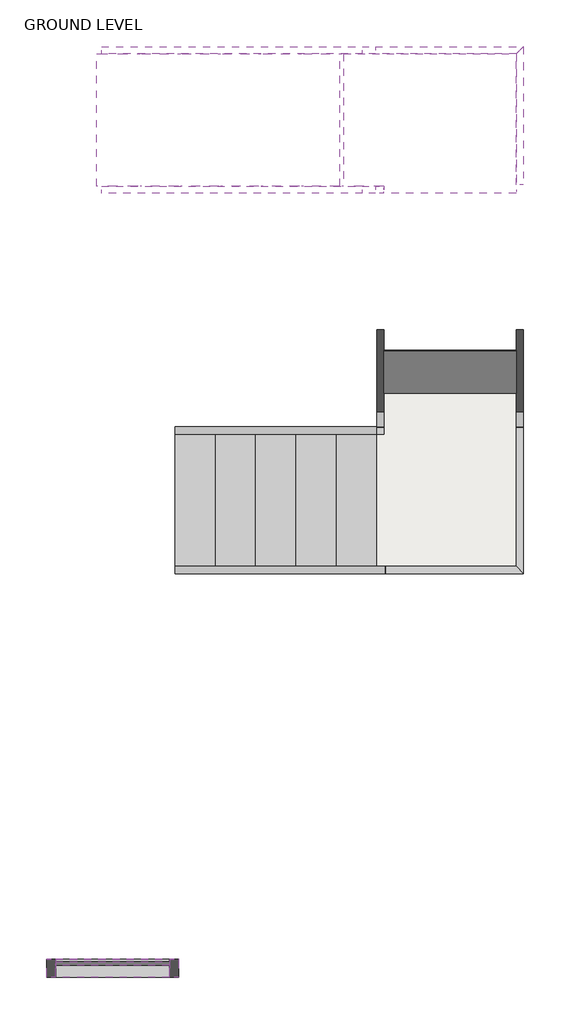
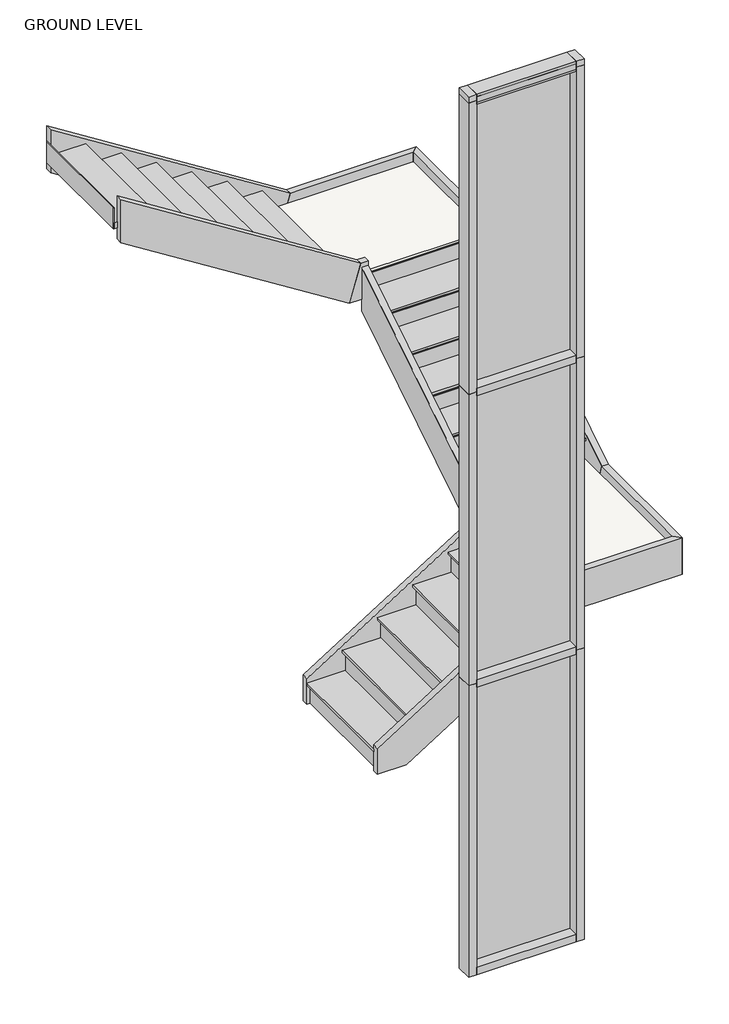
# One storey, incomplete: 25 members, 3 plates, 3 stair flights, 2 slabs.
"""IFC4 building model written with IfcOpenShell, lengths in millimetres."""

from ifc_helpers import new_model, si_unit, frame, origin, place, context, project, spatial, polyline, outline, extrude, faceted_brep, transform, mapped, element, save
from components import member_429f6687, member_18a184ad, member_ee409385, member_e0baf447, system_panel_glazed_7e875482, system_panel_glazed_4ec892b8, non_monolithic_landing_614a383d, non_monolithic_landing_589093d1, stair_flight_883e4480, stair_flight_150202ba, stair_flight_54ffcc7a

model = new_model("IFC4")

# Units and contexts
model_context = context("Model", 3, world=origin())
ifc_project = project(units=[si_unit("LENGTHUNIT", "METRE", prefix="MILLI")], contexts=[model_context])

# Site, building, storey
site = spatial("IfcSite", under=ifc_project)
building = spatial("IfcBuilding", under=site)
storey = spatial("IfcBuildingStorey", under=building, Name="GROUND LEVEL", Elevation=0.0)

# Members
placement = place(None, origin())
member_shape = member_429f6687(model_context)
element("IfcMember", 1, ObjectType="Rectangular Mullion : 2.5\" x 5\" rectangular", at=placement, inside=storey, context=model_context, shape_type="MappedRepresentation", body=[
    mapped(member_shape, transform((7470.37371, -13500.720363, 7669.779075), x_axis=(0.0, 0.0, 1.0), y_axis=(0.0, -1.0, 0.0), z_axis=(1.0, 0.0, 0.0))),
])
element("IfcMember", 2, ObjectType="Rectangular Mullion : 2.5\" x 5\" rectangular", at=placement, inside=storey, context=model_context, shape_type="MappedRepresentation", body=[
    mapped(member_shape, transform((6682.97371, -13500.720363, 304.8), x_axis=(0.0, 0.0, -1.0), y_axis=(0.0, -1.0, 0.0), z_axis=(-1.0, 0.0, 0.0))),
])
member_2_shape = member_18a184ad(model_context)
element("IfcMember", 3, ObjectType="Rectangular Mullion : 2.5\" x 5\" rectangular", at=placement, inside=storey, context=model_context, shape_type="MappedRepresentation", body=[
    mapped(member_2_shape, transform((7470.37371, -13500.720363, 2743.2), x_axis=(0.0, 0.0, 1.0), y_axis=(0.0, -1.0, 0.0), z_axis=(1.0, 0.0, 0.0))),
])
element("IfcMember", 4, ObjectType="Rectangular Mullion : 2.5\" x 5\" rectangular", at=placement, inside=storey, context=model_context, shape_type="MappedRepresentation", body=[
    mapped(member_2_shape, transform((7470.37371, -13500.720363, 5181.6), x_axis=(0.0, 0.0, 1.0), y_axis=(0.0, -1.0, 0.0), z_axis=(1.0, 0.0, 0.0))),
])
element("IfcMember", 5, ObjectType="Rectangular Mullion : 2.5\" x 5\" rectangular", at=placement, inside=storey, context=model_context, shape_type="MappedRepresentation", body=[
    mapped(member_2_shape, transform((7470.37371, -13500.720363, 7620.0), x_axis=(0.0, 0.0, 1.0), y_axis=(0.0, -1.0, 0.0), z_axis=(1.0, 0.0, 0.0))),
])
member_3_shape = member_ee409385(model_context)
element("IfcMember", 6, ObjectType="Rectangular Mullion : 2.5\" x 5\" rectangular", at=placement, inside=storey, context=model_context, shape_type="MappedRepresentation", body=[
    mapped(member_3_shape, transform((7533.87371, -13500.720363, 304.8), x_axis=(1.0, 0.0, 0.0), y_axis=(0.0, -1.0, 0.0), z_axis=(0.0, 0.0, -1.0))),
])
element("IfcMember", 7, ObjectType="Rectangular Mullion : 2.5\" x 5\" rectangular", at=placement, inside=storey, context=model_context, shape_type="MappedRepresentation", body=[
    mapped(member_3_shape, transform((6619.47371, -13500.720363, 2743.2), x_axis=(-1.0, 0.0, 0.0), y_axis=(0.0, -1.0, 0.0), z_axis=(0.0, 0.0, 1.0))),
])
element("IfcMember", 8, ObjectType="Rectangular Mullion : 2.5\" x 5\" rectangular", at=placement, inside=storey, context=model_context, shape_type="MappedRepresentation", body=[
    mapped(member_3_shape, transform((7533.87371, -13500.720363, 2743.2), x_axis=(1.0, 0.0, 0.0), y_axis=(0.0, -1.0, 0.0), z_axis=(0.0, 0.0, -1.0))),
])
element("IfcMember", 9, ObjectType="Rectangular Mullion : 2.5\" x 5\" rectangular", at=placement, inside=storey, context=model_context, shape_type="MappedRepresentation", body=[
    mapped(member_3_shape, transform((7533.87371, -13500.720363, 5181.6), x_axis=(1.0, 0.0, 0.0), y_axis=(0.0, -1.0, 0.0), z_axis=(0.0, 0.0, -1.0))),
])
element("IfcMember", 10, ObjectType="Rectangular Mullion : 2.5\" x 5\" rectangular", at=placement, inside=storey, context=model_context, shape_type="MappedRepresentation", body=[
    mapped(member_3_shape, transform((6619.47371, -13500.720363, 5181.6), x_axis=(-1.0, 0.0, 0.0), y_axis=(0.0, -1.0, 0.0), z_axis=(0.0, 0.0, 1.0))),
])
element("IfcMember", 11, ObjectType="Rectangular Mullion : 2.5\" x 5\" rectangular", at=placement, inside=storey, context=model_context, shape_type="MappedRepresentation", body=[
    mapped(member_3_shape, transform((6619.47371, -13500.720363, 7620.0), x_axis=(-1.0, 0.0, 0.0), y_axis=(0.0, -1.0, 0.0), z_axis=(0.0, 0.0, 1.0))),
])
member_4_shape = member_e0baf447(model_context)
element("IfcMember", 12, ObjectType="Rectangular Mullion : 2.5\" x 5\" rectangular", at=placement, inside=storey, context=model_context, shape_type="MappedRepresentation", body=[
    mapped(member_4_shape, transform((6619.47371, -13500.720363, 7669.779075), x_axis=(-1.0, 0.0, 0.0), y_axis=(0.0, -1.0, 0.0), z_axis=(0.0, 0.0, 1.0))),
])
element("IfcMember", 13, ObjectType="Rectangular Mullion : 2.5\" x 5\" rectangular", at=placement, inside=storey, context=model_context, shape_type="MappedRepresentation", body=[
    mapped(member_4_shape, transform((7533.87371, -13500.720363, 7620.0), x_axis=(1.0, 0.0, 0.0), y_axis=(0.0, -1.0, 0.0), z_axis=(0.0, 0.0, -1.0))),
])
element("IfcMember", 14, ObjectType="Stringer - 2\" Width", at=placement, inside=storey, context=model_context, shape_type="SweptSolid", body=[
    extrude(outline(polyline([(1888.9578947, 8807.4975826), (2193.7578947, 8895.691591), (3390.8812147, 7000.2463344), (3030.3797357, 7000.2463344), (1888.9578947, 8807.4975826)])), frame((0.0, -8140.7746824, 0.0), z_axis=(0.0, 1.0, 0.0), x_axis=(0.0, 0.0, 1.0)), (0.0, 0.0, 1.0), 50.8),
])
element("IfcMember", 15, ObjectType="Stringer - 2\" Width", at=placement, inside=storey, context=model_context, shape_type="SweptSolid", body=[
    extrude(outline(polyline([(1888.9578947, 8807.4975826), (2193.7578947, 8895.691591), (3390.8812147, 7000.2463344), (3030.3797357, 7000.2463344), (1888.9578947, 8807.4975826)])), frame((0.0, -7175.5746824, 0.0), z_axis=(0.0, 1.0, 0.0), x_axis=(0.0, 0.0, 1.0)), (0.0, 0.0, 1.0), 50.8),
])
element("IfcMember", 16, ObjectType="Stringer - 2\" Width", at=placement, inside=storey, context=model_context, shape_type="SweptSolid", body=[
    extrude(outline(polyline([(-9668.6259307, 830.1789474), (-9756.819939, 1134.9789474), (-8140.7746824, 2155.6391095), (-8140.7746824, 1795.1376305), (-9668.6259307, 830.1789474)])), frame((8906.0423568, 0.0, 0.0), z_axis=(1.0, 0.0, 0.0), x_axis=(0.0, 1.0, 0.0)), (0.0, 0.0, 1.0), 50.8),
])
element("IfcMember", 17, ObjectType="Stringer - 2\" Width", at=placement, inside=storey, context=model_context, shape_type="SweptSolid", body=[
    extrude(outline(polyline([(-9668.6259307, 830.1789474), (-9756.819939, 1134.9789474), (-8080.419939, 2193.7578947), (-7992.2259307, 1888.9578947), (-9668.6259307, 830.1789474)])), frame((9871.2423568, 0.0, 0.0), z_axis=(1.0, 0.0, 0.0), x_axis=(0.0, 1.0, 0.0)), (0.0, 0.0, 1.0), 50.8),
])
element("IfcMember", 18, ObjectType="Stringer - 2\" Width", at=placement, inside=storey, context=model_context, shape_type="SweptSolid", body=[
    extrude(outline(polyline([(2193.7578947, 8895.691591), (1888.9578947, 8807.4975826), (1888.9578947, 8956.8423568), (2193.7578947, 8956.8423568), (2193.7578947, 8895.691591)])), frame((0.0, -8140.7746824, 0.0), z_axis=(0.0, 1.0, 0.0), x_axis=(0.0, 0.0, 1.0)), (0.0, 0.0, 1.0), 50.8),
])
element("IfcMember", 19, ObjectType="Stringer - 2\" Width", at=placement, inside=storey, context=model_context, shape_type="Brep", body=[
    faceted_brep([(9871.2423568, -8080.419939, 2193.7578947), (9922.0423568, -8080.419939, 2193.7578947), (9922.0423568, -7124.7746824, 2193.7578947), (9871.2423568, -7175.5746824, 2193.7578947), (9871.2423568, -7992.2259307, 1888.9578947), (9871.2423568, -7175.5746824, 1888.9578947), (9922.0423568, -7992.2259307, 1888.9578947), (9922.0423568, -7124.7746824, 1888.9578947)], [[[0, 1, 2, 3]], [[4, 0, 3, 5]], [[6, 4, 5, 7]], [[1, 6, 7, 2]], [[1, 0, 4, 6]], [[2, 7, 5, 3]]]),
])
element("IfcMember", 20, ObjectType="Stringer - 2\" Width", at=placement, inside=storey, context=model_context, shape_type="Brep", body=[
    faceted_brep([(9871.2423568, -7175.5746824, 2193.7578947), (9922.0423568, -7124.7746824, 2193.7578947), (8895.691591, -7124.7746824, 2193.7578947), (8895.691591, -7175.5746824, 2193.7578947), (9871.2423568, -7175.5746824, 1888.9578947), (8807.4975826, -7175.5746824, 1888.9578947), (9922.0423568, -7124.7746824, 1888.9578947), (8807.4975826, -7124.7746824, 1888.9578947)], [[[0, 1, 2, 3]], [[4, 0, 3, 5]], [[6, 4, 5, 7]], [[1, 6, 7, 2]], [[1, 0, 4, 6]], [[2, 7, 5, 3]]]),
])
element("IfcMember", 21, ObjectType="Stringer - 2\" Width", at=placement, inside=storey, context=model_context, shape_type="SweptSolid", body=[
    extrude(outline(polyline([(214.5443726, 7509.0423568), (0.0, 7509.0423568), (0.0, 7740.1411085), (736.3586831, 8906.0423568), (1096.8601621, 8906.0423568), (214.5443726, 7509.0423568)])), frame((0.0, -9806.2073314, 0.0), z_axis=(0.0, 1.0, 0.0), x_axis=(0.0, 0.0, 1.0)), (0.0, 0.0, 1.0), 50.8),
])
element("IfcMember", 22, ObjectType="Stringer - 2\" Width", at=placement, inside=storey, context=model_context, shape_type="SweptSolid", body=[
    extrude(outline(polyline([(214.5443726, 7509.0423568), (0.0, 7509.0423568), (0.0, 7740.1411085), (830.1789474, 9054.5911085), (1134.9789474, 8966.3971001), (214.5443726, 7509.0423568)])), frame((0.0, -10771.4073314, 0.0), z_axis=(0.0, 1.0, 0.0), x_axis=(0.0, 0.0, 1.0)), (0.0, 0.0, 1.0), 50.8),
])
element("IfcMember", 23, ObjectType="Stringer - 2\" Width", at=placement, inside=storey, context=model_context, shape_type="SweptSolid", body=[
    extrude(outline(polyline([(-9756.819939, 1134.9789474), (-9668.6259307, 830.1789474), (-9806.2073314, 830.1789474), (-9806.2073314, 1134.9789474), (-9756.819939, 1134.9789474)])), frame((8906.0423568, 0.0, 0.0), z_axis=(1.0, 0.0, 0.0), x_axis=(0.0, 1.0, 0.0)), (0.0, 0.0, 1.0), 50.8),
])
element("IfcMember", 24, ObjectType="Stringer - 2\" Width", at=placement, inside=storey, context=model_context, shape_type="Brep", body=[
    faceted_brep([(8966.3971001, -10720.6073314, 1134.9789474), (8966.3971001, -10771.4073314, 1134.9789474), (9922.0423568, -10771.4073314, 1134.9789474), (9871.2423568, -10720.6073314, 1134.9789474), (9054.5911085, -10720.6073314, 830.1789474), (9871.2423568, -10720.6073314, 830.1789474), (9054.5911085, -10771.4073314, 830.1789474), (9922.0423568, -10771.4073314, 830.1789474)], [[[0, 1, 2, 3]], [[4, 0, 3, 5]], [[6, 4, 5, 7]], [[1, 6, 7, 2]], [[1, 0, 4, 6]], [[2, 7, 5, 3]]]),
])
element("IfcMember", 25, ObjectType="Stringer - 2\" Width", at=placement, inside=storey, context=model_context, shape_type="Brep", body=[
    faceted_brep([(9871.2423568, -10720.6073314, 1134.9789474), (9922.0423568, -10771.4073314, 1134.9789474), (9922.0423568, -9756.819939, 1134.9789474), (9871.2423568, -9756.819939, 1134.9789474), (9871.2423568, -10720.6073314, 830.1789474), (9871.2423568, -9668.6259307, 830.1789474), (9922.0423568, -10771.4073314, 830.1789474), (9922.0423568, -9668.6259307, 830.1789474)], [[[0, 1, 2, 3]], [[4, 0, 3, 5]], [[6, 4, 5, 7]], [[1, 6, 7, 2]], [[1, 0, 4, 6]], [[2, 7, 5, 3]]]),
])

# Plates
system_panel_glazed_shape = system_panel_glazed_7e875482(model_context)
element("IfcPlate", 26, ObjectType="System Panel : Glazed", at=placement, inside=storey, context=model_context, shape_type="MappedRepresentation", body=[
    mapped(system_panel_glazed_shape, transform((7076.67371, -13500.720363, 368.3), x_axis=(1.0, 0.0, 0.0), y_axis=(0.0, 1.0, 0.0), z_axis=(0.0, 0.0, 1.0))),
])
system_panel_glazed_2_shape = system_panel_glazed_4ec892b8(model_context)
element("IfcPlate", 27, ObjectType="System Panel : Glazed", at=placement, inside=storey, context=model_context, shape_type="MappedRepresentation", body=[
    mapped(system_panel_glazed_2_shape, transform((7076.67371, -13500.720363, 2774.95), x_axis=(1.0, 0.0, 0.0), y_axis=(0.0, 1.0, 0.0), z_axis=(0.0, 0.0, 1.0))),
])
element("IfcPlate", 28, ObjectType="System Panel : Glazed", at=placement, inside=storey, context=model_context, shape_type="MappedRepresentation", body=[
    mapped(system_panel_glazed_2_shape, transform((7076.67371, -13500.720363, 5213.35), x_axis=(1.0, 0.0, 0.0), y_axis=(0.0, 1.0, 0.0), z_axis=(0.0, 0.0, 1.0))),
])

# Slabs
non_monolithic_landing_shape = non_monolithic_landing_614a383d(model_context)
element("IfcSlab", 29, ObjectType="Non-Monolithic Landing", at=placement, inside=storey, context=model_context, shape_type="MappedRepresentation", body=[
    mapped(non_monolithic_landing_shape, transform((0.0, 0.0, 0.0), x_axis=(1.0, 0.0, 0.0), y_axis=(0.0, 1.0, 0.0), z_axis=(0.0, 0.0, 1.0))),
])
non_monolithic_landing_2_shape = non_monolithic_landing_589093d1(model_context)
element("IfcSlab", 30, ObjectType="Non-Monolithic Landing", at=placement, inside=storey, context=model_context, shape_type="MappedRepresentation", body=[
    mapped(non_monolithic_landing_2_shape, transform((0.0, 0.0, 0.0), x_axis=(1.0, 0.0, 0.0), y_axis=(0.0, 1.0, 0.0), z_axis=(0.0, 0.0, 1.0))),
])

# Stair flights
stair_flight_shape = stair_flight_883e4480(model_context)
element("IfcStairFlight", 31, ObjectType="2\" Tread 1\" Nosing 1/4\" Riser", at=placement, inside=storey, context=model_context, shape_type="MappedRepresentation", body=[
    mapped(stair_flight_shape, transform((0.0, 0.0, 0.0), x_axis=(1.0, 0.0, 0.0), y_axis=(0.0, 1.0, 0.0), z_axis=(0.0, 0.0, 1.0))),
])
stair_flight_2_shape = stair_flight_150202ba(model_context)
element("IfcStairFlight", 32, ObjectType="2\" Tread 1\" Nosing 1/4\" Riser", at=placement, inside=storey, context=model_context, shape_type="MappedRepresentation", body=[
    mapped(stair_flight_2_shape, transform((0.0, 0.0, 0.0), x_axis=(1.0, 0.0, 0.0), y_axis=(0.0, 1.0, 0.0), z_axis=(0.0, 0.0, 1.0))),
])
stair_flight_3_shape = stair_flight_54ffcc7a(model_context)
element("IfcStairFlight", 33, ObjectType="2\" Tread 1\" Nosing 1/4\" Riser", at=placement, inside=storey, context=model_context, shape_type="MappedRepresentation", body=[
    mapped(stair_flight_3_shape, transform((0.0, 0.0, 0.0), x_axis=(1.0, 0.0, 0.0), y_axis=(0.0, 1.0, 0.0), z_axis=(0.0, 0.0, 1.0))),
])

save(model, "model.ifc")

# Revit data of these elements
# Type "Rectangular Mullion : 2.5\" x 5\" rectangular"
#   built-in parameter 1007304 = 0.416667 (stored number, unit not read)
#   built-in parameter 1007301 = 0.104167 (stored number, unit not read)
#   built-in parameter 1007300 = 0.104167 (stored number, unit not read)
# Type "System Panel : Glazed"
#   Construction Type Id = "GSP4R"
#   Analytic Construction = "1/8 in Pilkington single glazing"
#   Visual Light Transmittance = 0.9
#   Solar Heat Gain Coefficient = 0.86
#   Heat Transfer Coefficient (U) = 1.18115 BTU/(h·ft²·°F)
#   Define Thermal Properties by = 1
# Elements 1, 2, 3, 4, 5, 6, 7, 8, 9, 10, 11, 12, 13 (IfcMember, "Rectangular Mullion : 2.5\" x 5\" rectangular")
#   Phase Created = New Construction
#   Materials on its faces: "BLACK MATERIAL"
# Elements 14, 16, 21, 22, 23, 24 (IfcMember, "Stringer - 2\" Width")
#   Phase Created = New Construction
#   Materials on its faces: "MARBLE STAIRS 6\""
# Elements 15, 17, 18, 19, 20, 25 (IfcMember, "Stringer - 2\" Width")
#   Phase Created = New Construction
# Elements 26, 27, 28 (IfcPlate, "System Panel : Glazed")
#   Phase Created = New Construction
#   Materials on its faces: "Glass"
# Elements 29, 30 (IfcSlab, "Non-Monolithic Landing")
#   Phase Created = New Construction
#   Materials on its faces: "MARBLE STAIRS 6\""
# Elements 31, 32, 33 (IfcStairFlight, "2\" Tread 1\" Nosing 1/4\" Riser")
#   Phase Created = New Construction
#   Materials on its faces: "MARBLE STAIRS 6\""
# Materials
#   "BLACK MATERIAL": class "Generic", colour RGB 120 120 120, transparency 0, Cost = 0
#   "MARBLE STAIRS 6\"": class "Generic", colour RGB 120 120 120, transparency 0, Cost = 0
#   "Glass": class "Glass", colour RGB 0 128 192, transparency 0.75, Description = "Soda Lime Glass", Cost = 0
